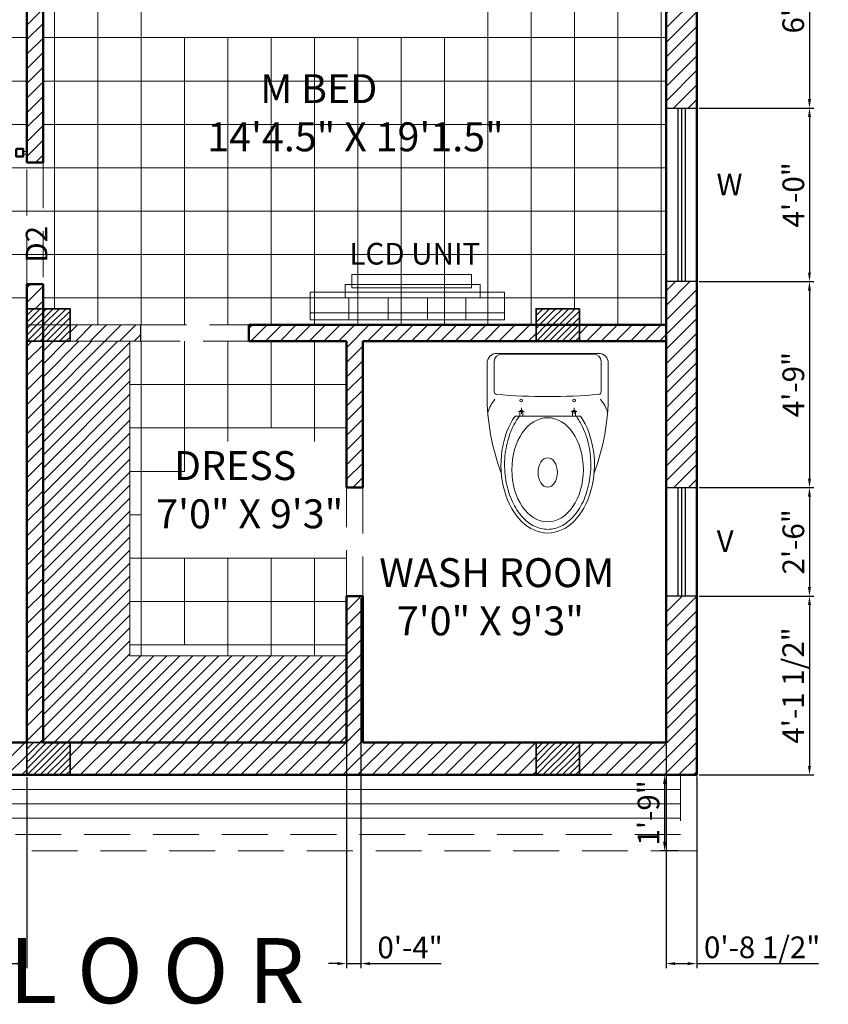
# Model space of a CAD drawing. Units: millimetres. Extents: x 225995 to 227247, y 225507 to 226008.
# Tile 4 of 23: x 226378 to 226602, y 225507 to 225780. Entities that reach past the tile are written whole.
import ezdxf

# ---------------------------------------------------------------- set-up
doc = ezdxf.new("R2010")
doc.units = ezdxf.units.MM
doc.linetypes.add('DASHED', pattern=[19.05, 12.7, -6.35])
for name, color, linetype, lineweight in [('A-ANNO-DIMS', 2, 'Continuous', 18), ('A-ANNO-TEXT', 3, 'Continuous', 18), ('A-AREA-IDEN', 30, 'Continuous', 18), ('A-COLS', 40, 'Continuous', 35), ('A-FLOR-FIXT', 8, 'Continuous', 18), ('A-FLOR-PATT', 8, 'Continuous', 13), ('A-FURN', 9, 'Continuous', 18), ('A-GLAZ', 4, 'Continuous', 25), ('A-WALL', 7, 'Continuous', 50), ('A-WALL-OVHD', 1, 'DASHED', 18), ('A-WALL-PATT', 8, 'Continuous', 13)]:
    doc.layers.add(name, color=color, linetype=linetype, lineweight=lineweight)
doc.styles.get("Standard").update_dxf_attribs({"font": 'arial.ttf'})
doc.dimstyles.new('ISO-25', dxfattribs={"dimtxt": 6, "dimasz": 2.5, "dimexe": 1.25, "dimexo": 0.625, "dimtad": 1, "dimdec": 0, "dimlunit": 3, "dimtxsty": 'Standard', "dimcen": 2.5, "dimadec": 0, "dimazin": 0, "dimtfac": 1, "dimtdec": 0, "dimtmove": 0, "dimatfit": 3, "dimfxl": 1, "dimarcsym": 0})
pattern_1 = [(45, (141, 0), (-0.898025612, 0.898025612), [])]
pattern_2 = [(45, (0, -120), (-0.898025612, 0.898025612), [])]
pattern_3 = [(45, (141, -120), (-0.898025612, 0.898025612), [])]

# ---------------------------------------------------------------- blocks, each defined once
blk = doc.blocks.new('A$C005B7AE8')
for p, q in [((0.46, 0.74), (0.04, 0.74)), ((0.44, 0.7369), (0.06, 0.7369)), ((0, 0.7), (0, 0.569)), ((0.03, 0.7069), (0.03, 0.5811)), ((0.47, 0.7069), (0.47, 0.5811)), ((0.5, 0.7), (0.5, 0.569)), ((0.1298, 0.5004), (0.1534, 0.5004)), ((0.1356, 0.482), (0.1356, 0.5012)), ((0.1415, 0.4917), (0.1415, 0.5154)), ((0.1478, 0.5012), (0.1478, 0.482)), ((0.3702, 0.5004), (0.3466, 0.5004)), ((0.3522, 0.5012), (0.3522, 0.482)), ((0.3585, 0.4917), (0.3585, 0.5154)), ((0.3644, 0.482), (0.3644, 0.5012)), ((0.3847, 0.482), (0.1153, 0.482))]:
    blk.add_line(p, q)
for centre in [(0.1408, 0.546), (0.3592, 0.546)]:
    blk.add_circle(centre, 0.00582)
for centre, radius, start, end in [((0.04, 0.7), 0.04, 90, 180), ((0.06, 0.7069), 0.03, 90, 180), ((0.44, 0.7069), 0.03, 0, 90), ((0.46, 0.7), 0.04, 0, 90), ((0.9162, 0.5698), 0.9162, 179.9528, 200.6123), ((0.04, 0.5811), 0.01, 180, 265.0115), ((0.25, 2.987), 2.425, 265.0115, 274.9885), ((-0.4162, 0.5698), 0.9162, 339.3877, 0.0472), ((0.46, 0.5811), 0.01, 274.9885, 0), ((0.1538, 0.4498), 0.1579, 140.1815, 162.8478), ((0.3462, 0.4498), 0.1579, 17.1522, 39.8185), ((0.1417, 0.5006), 0.00615, 5.1568, 174.8432), ((0.3583, 0.5006), 0.00615, 5.1568, 174.8432)]:
    blk.add_arc(centre, radius, start, end)
blk.add_ellipse((0.25, 0.281), major_axis=(0, -0.281), ratio=0.685919, start_param=3.915332, end_param=8.651039)
for centre, major_axis, ratio in [((0.2497, 0.2607), (0, -0.2144), 0.687861), ((0.25, 0.2496), (0, -0.0607), 0.657164)]:
    blk.add_ellipse(centre, major_axis=major_axis, ratio=ratio)
blk.add_open_spline([(0.133, 0.4806), (0.1233, 0.4673), (0.1192, 0.4608), (0.109, 0.4431), (0.1032, 0.4313), (0.0931, 0.4064), (0.0887, 0.3933), (0.0814, 0.3662), (0.0785, 0.3521), (0.0743, 0.3236), (0.073, 0.3091), (0.072, 0.2798), (0.0723, 0.2652), (0.0746, 0.2361), (0.0765, 0.2217), (0.0819, 0.1936), (0.0854, 0.1799), (0.0938, 0.1536), (0.0988, 0.141), (0.1099, 0.1171), (0.1162, 0.1059), (0.1297, 0.0851), (0.137, 0.0756), (0.1525, 0.0585), (0.1607, 0.0509), (0.1776, 0.0379), (0.1863, 0.0325), (0.2042, 0.0237), (0.2132, 0.0204), (0.2316, 0.0161), (0.2408, 0.015), (0.2593, 0.015), (0.2685, 0.0161), (0.2868, 0.0205), (0.2959, 0.0237), (0.3137, 0.0325), (0.3225, 0.0379), (0.3394, 0.051), (0.3475, 0.0586), (0.363, 0.0756), (0.3703, 0.0852), (0.3839, 0.1059), (0.3901, 0.1172), (0.4013, 0.141), (0.4062, 0.1537), (0.4146, 0.18), (0.4181, 0.1937), (0.4235, 0.2218), (0.4255, 0.2362), (0.4277, 0.2653), (0.428, 0.2799), (0.427, 0.3091), (0.4257, 0.3237), (0.4215, 0.3522), (0.4186, 0.3662), (0.4113, 0.3933), (0.4069, 0.4064), (0.3967, 0.4313), (0.391, 0.4432), (0.3808, 0.4609), (0.3767, 0.4673), (0.3673, 0.4823)], degree=3, knots=[3.915332, 3.915332, 3.915332, 3.915332, 4.014441, 4.014441, 4.176505, 4.176505, 4.338569, 4.338569, 4.500633, 4.500633, 4.662697, 4.662697, 4.824761, 4.824761, 4.986825, 4.986825, 5.148889, 5.148889, 5.310953, 5.310953, 5.473017, 5.473017, 5.635081, 5.635081, 5.797146, 5.797146, 5.95921, 5.95921, 6.121274, 6.121274, 6.283338, 6.283338, 6.445402, 6.445402, 6.607466, 6.607466, 6.76953, 6.76953, 6.931594, 6.931594, 7.093658, 7.093658, 7.255722, 7.255722, 7.417786, 7.417786, 7.57985, 7.57985, 7.741915, 7.741915, 7.903979, 7.903979, 8.066043, 8.066043, 8.228107, 8.228107, 8.390171, 8.390171, 8.552235, 8.552235, 8.651039, 8.651039, 8.651039, 8.651039])
blk = doc.blocks.new('*D67')
at = {"layer": 'A-ANNO-DIMS', "color": 0, "lineweight": -2, "transparency": 16777216}
for p, q in [((226560.75, 225570.77), (226555.72, 225570.77)), ((226556.97, 225568.27), (226556.97, 225552.27)), ((226560.75, 225549.77), (226555.72, 225549.77))]:
    blk.add_line(p, q, dxfattribs=at)
at = {"layer": 'A-ANNO-DIMS', "color": 0, "transparency": 16777216}
for points in [[(226556.55, 225568.27), (226557.38, 225568.27), (226556.97, 225570.77)], [(226556.55, 225552.27), (226557.38, 225552.27), (226556.97, 225549.77)]]:
    blk.add_solid(points, dxfattribs=at)
at = {"layer": 'Defpoints', "color": 0, "transparency": 16777216}
for p in [(226561.38, 225570.77), (226556.97, 225549.77), (226561.38, 225549.77)]:
    blk.add_point(p, dxfattribs=at)
at = {"layer": 'A-ANNO-DIMS', "color": 0, "transparency": 16777216, "insert": (226553.28, 225560.27), "char_height": 6, "attachment_point": 5, "rotation": 90}
blk.add_mtext('1\'-9"', dxfattribs=at)
blk = doc.blocks.new('*D91')
at = {"layer": 'A-ANNO-DIMS', "color": 0, "lineweight": -2, "transparency": 16777216}
for p, q in [((226557.38, 225579.15), (226557.38, 225517.32)), ((226565.88, 225570.15), (226565.88, 225517.32)), ((226559.88, 225518.57), (226563.38, 225518.57)), ((226565.88, 225518.57), (226599.56, 225518.57))]:
    blk.add_line(p, q, dxfattribs=at)
at = {"layer": 'A-ANNO-DIMS', "color": 0, "transparency": 16777216}
for points in [[(226559.88, 225518.99), (226559.88, 225518.16), (226557.38, 225518.57)], [(226563.38, 225518.99), (226563.38, 225518.16), (226565.88, 225518.57)]]:
    blk.add_solid(points, dxfattribs=at)
at = {"layer": 'Defpoints', "color": 0, "transparency": 16777216}
for p in [(226557.38, 225579.77), (226565.88, 225570.77), (226565.88, 225518.57)]:
    blk.add_point(p, dxfattribs=at)
at = {"layer": 'A-ANNO-DIMS', "color": 0, "transparency": 16777216, "insert": (226583.97, 225522.3), "char_height": 6, "attachment_point": 5}
blk.add_mtext('0\'-8 1/2"', dxfattribs=at)
blk = doc.blocks.new('*D92')
at = {"layer": 'A-ANNO-DIMS', "color": 0, "lineweight": -2, "transparency": 16777216}
for p, q in [((226468.88, 225619.65), (226468.88, 225517.32)), ((226472.89, 225619.65), (226472.89, 225517.32)), ((226466.38, 225518.57), (226463.88, 225518.57)), ((226468.88, 225518.57), (226472.89, 225518.57)), ((226475.39, 225518.57), (226495.09, 225518.57))]:
    blk.add_line(p, q, dxfattribs=at)
at = {"layer": 'A-ANNO-DIMS', "color": 0, "transparency": 16777216}
for points in [[(226466.38, 225518.99), (226466.38, 225518.16), (226468.88, 225518.57)], [(226475.39, 225518.99), (226475.39, 225518.16), (226472.89, 225518.57)]]:
    blk.add_solid(points, dxfattribs=at)
at = {"layer": 'Defpoints', "color": 0, "transparency": 16777216}
for p in [(226468.88, 225620.27), (226472.89, 225620.27), (226472.89, 225518.57)]:
    blk.add_point(p, dxfattribs=at)
at = {"layer": 'A-ANNO-DIMS', "color": 0, "transparency": 16777216, "insert": (226486.49, 225522.26), "char_height": 6, "attachment_point": 5}
blk.add_mtext('0\'-4"', dxfattribs=at)
blk = doc.blocks.new('*D101')
at = {"layer": 'A-ANNO-DIMS', "color": 0, "lineweight": -2, "transparency": 16777216}
for p, q in [((226566.5, 225828.77), (226598.33, 225828.77)), ((226597.08, 225826.27), (226597.08, 225757.77)), ((226566.5, 225755.27), (226598.33, 225755.27))]:
    blk.add_line(p, q, dxfattribs=at)
at = {"layer": 'A-ANNO-DIMS', "color": 0, "transparency": 16777216}
for points in [[(226596.66, 225826.27), (226597.49, 225826.27), (226597.08, 225828.77)], [(226596.66, 225757.77), (226597.49, 225757.77), (226597.08, 225755.27)]]:
    blk.add_solid(points, dxfattribs=at)
at = {"layer": 'Defpoints', "color": 0, "transparency": 16777216}
for p in [(226565.88, 225828.77), (226565.88, 225755.27), (226597.08, 225755.27)]:
    blk.add_point(p, dxfattribs=at)
at = {"layer": 'A-ANNO-DIMS', "color": 0, "transparency": 16777216, "insert": (226593.35, 225792.02), "char_height": 6, "attachment_point": 5, "rotation": 90}
blk.add_mtext('6\'-1 1/2"', dxfattribs=at)
blk = doc.blocks.new('*D102')
at = {"layer": 'A-ANNO-DIMS', "color": 0, "lineweight": -2, "transparency": 16777216}
for p, q in [((226566.5, 225755.27), (226598.33, 225755.27)), ((226597.08, 225752.77), (226597.08, 225709.77)), ((226566.5, 225707.27), (226598.33, 225707.27))]:
    blk.add_line(p, q, dxfattribs=at)
at = {"layer": 'A-ANNO-DIMS', "color": 0, "transparency": 16777216}
for points in [[(226596.66, 225752.77), (226597.49, 225752.77), (226597.08, 225755.27)], [(226596.66, 225709.77), (226597.49, 225709.77), (226597.08, 225707.27)]]:
    blk.add_solid(points, dxfattribs=at)
at = {"layer": 'Defpoints', "color": 0, "transparency": 16777216}
for p in [(226565.88, 225755.27), (226565.88, 225707.27), (226597.08, 225707.27)]:
    blk.add_point(p, dxfattribs=at)
at = {"layer": 'A-ANNO-DIMS', "color": 0, "transparency": 16777216, "insert": (226593.39, 225731.27), "char_height": 6, "attachment_point": 5, "rotation": 90}
blk.add_mtext('4\'-0"', dxfattribs=at)
blk = doc.blocks.new('*D103')
at = {"layer": 'A-ANNO-DIMS', "color": 0, "lineweight": -2, "transparency": 16777216}
for p, q in [((226566.5, 225707.27), (226598.33, 225707.27)), ((226597.08, 225704.77), (226597.08, 225652.77)), ((226566.5, 225650.27), (226598.33, 225650.27))]:
    blk.add_line(p, q, dxfattribs=at)
at = {"layer": 'A-ANNO-DIMS', "color": 0, "transparency": 16777216}
for points in [[(226596.66, 225704.77), (226597.49, 225704.77), (226597.08, 225707.27)], [(226596.66, 225652.77), (226597.49, 225652.77), (226597.08, 225650.27)]]:
    blk.add_solid(points, dxfattribs=at)
at = {"layer": 'Defpoints', "color": 0, "transparency": 16777216}
for p in [(226565.88, 225707.27), (226565.88, 225650.27), (226597.08, 225650.27)]:
    blk.add_point(p, dxfattribs=at)
at = {"layer": 'A-ANNO-DIMS', "color": 0, "transparency": 16777216, "insert": (226593.39, 225678.77), "char_height": 6, "attachment_point": 5, "rotation": 90}
blk.add_mtext('4\'-9"', dxfattribs=at)
blk = doc.blocks.new('*D104')
at = {"layer": 'A-ANNO-DIMS', "color": 0, "lineweight": -2, "transparency": 16777216}
for p, q in [((226566.5, 225650.27), (226598.33, 225650.27)), ((226597.08, 225647.77), (226597.08, 225622.77)), ((226566.5, 225620.27), (226598.33, 225620.27))]:
    blk.add_line(p, q, dxfattribs=at)
at = {"layer": 'A-ANNO-DIMS', "color": 0, "transparency": 16777216}
for points in [[(226596.66, 225647.77), (226597.49, 225647.77), (226597.08, 225650.27)], [(226596.66, 225622.77), (226597.49, 225622.77), (226597.08, 225620.27)]]:
    blk.add_solid(points, dxfattribs=at)
at = {"layer": 'Defpoints', "color": 0, "transparency": 16777216}
for p in [(226565.88, 225650.27), (226565.88, 225620.27), (226597.08, 225620.27)]:
    blk.add_point(p, dxfattribs=at)
at = {"layer": 'A-ANNO-DIMS', "color": 0, "transparency": 16777216, "insert": (226593.39, 225635.27), "char_height": 6, "attachment_point": 5, "rotation": 90}
blk.add_mtext('2\'-6"', dxfattribs=at)
blk = doc.blocks.new('*D105')
at = {"layer": 'A-ANNO-DIMS', "color": 0, "lineweight": -2, "transparency": 16777216}
for p, q in [((226566.5, 225620.27), (226598.33, 225620.27)), ((226597.08, 225617.77), (226597.08, 225573.27)), ((226566.5, 225570.77), (226598.33, 225570.77))]:
    blk.add_line(p, q, dxfattribs=at)
at = {"layer": 'A-ANNO-DIMS', "color": 0, "transparency": 16777216}
for points in [[(226596.66, 225617.77), (226597.49, 225617.77), (226597.08, 225620.27)], [(226596.66, 225573.27), (226597.49, 225573.27), (226597.08, 225570.77)]]:
    blk.add_solid(points, dxfattribs=at)
at = {"layer": 'Defpoints', "color": 0, "transparency": 16777216}
for p in [(226565.88, 225620.27), (226565.88, 225570.77), (226597.08, 225570.77)]:
    blk.add_point(p, dxfattribs=at)
at = {"layer": 'A-ANNO-DIMS', "color": 0, "transparency": 16777216, "insert": (226593.35, 225595.52), "char_height": 6, "attachment_point": 5, "rotation": 90}
blk.add_mtext('4\'-1 1/2"', dxfattribs=at)
blk = doc.blocks.new('*D107')
at = {"layer": 'A-ANNO-DIMS', "color": 0, "lineweight": -2, "transparency": 16777216}
for p, q in [((226344.38, 225570.15), (226344.38, 225517.32)), ((226380.38, 225570.15), (226380.38, 225517.32)), ((226346.88, 225518.57), (226377.88, 225518.57))]:
    blk.add_line(p, q, dxfattribs=at)
at = {"layer": 'A-ANNO-DIMS', "color": 0, "transparency": 16777216}
for points in [[(226346.88, 225518.99), (226346.88, 225518.16), (226344.38, 225518.57)], [(226377.88, 225518.99), (226377.88, 225518.16), (226380.38, 225518.57)]]:
    blk.add_solid(points, dxfattribs=at)
at = {"layer": 'Defpoints', "color": 0, "transparency": 16777216}
for p in [(226344.38, 225570.77), (226380.38, 225570.77), (226380.38, 225518.57)]:
    blk.add_point(p, dxfattribs=at)
at = {"layer": 'A-ANNO-DIMS', "color": 0, "transparency": 16777216, "insert": (226362.38, 225522.26), "char_height": 6, "attachment_point": 5}
blk.add_mtext('3\'-0"', dxfattribs=at)

msp = doc.modelspace()

# ---------------------------------------------------------------- hatches: boundary and pattern name
at = {"layer": 'A-WALL-PATT'}
h = msp.add_hatch(dxfattribs=at)
h.set_pattern_fill('ANSI31', color=256, scale=0.9)
h.paths.add_polyline_path([(226565.88, 225828.77), (226557.38, 225828.77), (226557.38, 225755.27), (226565.88, 225755.27)])
h = msp.add_hatch(dxfattribs=at)
h.set_pattern_fill('ANSI31', color=256, scale=0.9)
h.paths.add_polyline_path([(226384.88, 225808.91), (226380.38, 225808.91), (226380.38, 225740.27), (226384.88, 225740.27)])
h = msp.add_hatch(dxfattribs=at)
h.set_pattern_fill('ANSI31', color=256, scale=0.9)
h.paths.add_polyline_path([(226565.88, 225707.27), (226557.38, 225707.27), (226557.38, 225695.27), (226533.38, 225695.27), (226533.38, 225690.77), (226557.38, 225690.77), (226557.38, 225650.27), (226565.88, 225650.27)])
h = msp.add_hatch(dxfattribs=at)
h.set_pattern_fill('ANSI31', color=256, scale=0.9)
h.paths.add_polyline_path([(226384.88, 225706.52), (226380.38, 225706.52), (226380.38, 225699.77), (226384.88, 225699.77)])
h = msp.add_hatch(dxfattribs=at)
h.set_pattern_fill('ANSI31', color=256, scale=0.4)
h.paths.add_polyline_path([(226384.88, 225699.77), (226380.38, 225699.77), (226380.38, 225695.27), (226384.88, 225695.27)])
h = msp.add_hatch(dxfattribs=at)
h.set_pattern_fill('ANSI31', color=256, scale=0.4)
h.paths.add_polyline_path([(226392.38, 225699.77), (226384.88, 225699.77), (226384.88, 225695.27), (226392.38, 225695.27)])
h = msp.add_hatch(dxfattribs=at)
h.set_pattern_fill('ANSI31', color=256, scale=0.4)
h.set_pattern_definition(pattern_1)
h.paths.add_polyline_path([(226525.88, 225699.77), (226521.38, 225699.77), (226521.38, 225695.27), (226525.88, 225695.27)])
h = msp.add_hatch(dxfattribs=at)
h.set_pattern_fill('ANSI31', color=256, scale=0.4)
h.set_pattern_definition(pattern_1)
h.paths.add_polyline_path([(226533.38, 225699.77), (226525.88, 225699.77), (226525.88, 225695.27), (226533.38, 225695.27)])
h = msp.add_hatch(dxfattribs=at)
h.set_pattern_fill('ANSI31', color=256, scale=0.4)
h.paths.add_polyline_path([(226384.88, 225695.27), (226380.38, 225695.27), (226380.38, 225690.77), (226384.88, 225690.77)])
h = msp.add_hatch(dxfattribs=at)
h.set_pattern_fill('ANSI31', color=256, scale=0.4)
h.paths.add_polyline_path([(226392.38, 225695.27), (226384.88, 225695.27), (226384.88, 225690.77), (226392.38, 225690.77)])
h = msp.add_hatch(dxfattribs=at)
h.set_pattern_fill('ANSI31', color=256, scale=0.9)
h.paths.add_polyline_path([(226411.88, 225695.27), (226392.38, 225695.27), (226392.38, 225690.77), (226411.88, 225690.77)])
h = msp.add_hatch(dxfattribs=at)
h.set_pattern_fill('ANSI31', color=256, scale=0.9)
h.paths.add_polyline_path([(226521.38, 225695.27), (226441.88, 225695.27), (226441.88, 225690.77), (226468.88, 225690.77), (226468.88, 225650.27), (226473.38, 225650.27), (226473.38, 225690.77), (226521.38, 225690.77)])
h = msp.add_hatch(dxfattribs=at)
h.set_pattern_fill('ANSI31', color=256, scale=0.4)
h.set_pattern_definition(pattern_1)
h.paths.add_polyline_path([(226525.88, 225695.27), (226521.38, 225695.27), (226521.38, 225690.77), (226525.88, 225690.77)])
h = msp.add_hatch(dxfattribs=at)
h.set_pattern_fill('ANSI31', color=256, scale=0.4)
h.set_pattern_definition(pattern_1)
h.paths.add_polyline_path([(226533.38, 225695.27), (226525.88, 225695.27), (226525.88, 225690.77), (226533.38, 225690.77)])
h = msp.add_hatch(dxfattribs=at)
h.set_pattern_fill('ANSI31', color=256, scale=0.9)
h.paths.add_polyline_path([(226384.88, 225690.77), (226380.38, 225690.77), (226380.38, 225579.77), (226384.88, 225579.77)])
h = msp.add_hatch(dxfattribs=at)
h.set_pattern_fill('ANSI31', color=256, scale=0.8)
h.paths.add_polyline_path([(226468.88, 225603.77), (226408.88, 225603.77), (226408.88, 225690.77), (226384.88, 225690.77), (226384.88, 225579.77), (226392.38, 225579.77), (226468.88, 225579.77)])
h = msp.add_hatch(dxfattribs=at)
h.set_pattern_fill('ANSI31', color=256, scale=0.9)
h.paths.add_polyline_path([(226521.38, 225579.77), (226473.38, 225579.77), (226473.38, 225620.27), (226468.88, 225620.27), (226468.88, 225579.77), (226392.38, 225579.77), (226392.38, 225570.77), (226521.38, 225570.77)])
h = msp.add_hatch(dxfattribs=at)
h.set_pattern_fill('ANSI31', color=256, scale=0.9)
h.paths.add_polyline_path([(226565.88, 225620.27), (226557.38, 225620.27), (226557.38, 225579.77), (226533.38, 225579.77), (226533.38, 225570.77), (226565.88, 225570.77)])
h = msp.add_hatch(dxfattribs=at)
h.set_pattern_fill('ANSI31', color=256, scale=0.9)
h.paths.add_polyline_path([(226380.38, 225579.77), (226344.38, 225579.77), (226344.38, 225570.77), (226380.38, 225570.77)])
h = msp.add_hatch(dxfattribs=at)
h.set_pattern_fill('ANSI31', color=256, scale=0.4)
h.set_pattern_definition(pattern_2)
h.paths.add_polyline_path([(226384.88, 225579.77), (226380.38, 225579.77), (226380.38, 225575.27), (226384.88, 225575.27)])
h = msp.add_hatch(dxfattribs=at)
h.set_pattern_fill('ANSI31', color=256, scale=0.4)
h.set_pattern_definition(pattern_2)
h.paths.add_polyline_path([(226392.38, 225579.77), (226384.88, 225579.77), (226384.88, 225575.27), (226392.38, 225575.27)])
h = msp.add_hatch(dxfattribs=at)
h.set_pattern_fill('ANSI31', color=256, scale=0.4)
h.set_pattern_definition(pattern_3)
h.paths.add_polyline_path([(226525.88, 225579.77), (226521.38, 225579.77), (226521.38, 225575.27), (226525.88, 225575.27)])
h = msp.add_hatch(dxfattribs=at)
h.set_pattern_fill('ANSI31', color=256, scale=0.4)
h.set_pattern_definition(pattern_3)
h.paths.add_polyline_path([(226533.38, 225579.77), (226525.88, 225579.77), (226525.88, 225575.27), (226533.38, 225575.27)])
h = msp.add_hatch(dxfattribs=at)
h.set_pattern_fill('ANSI31', color=256, scale=0.4)
h.set_pattern_definition(pattern_2)
h.paths.add_polyline_path([(226384.88, 225575.27), (226380.38, 225575.27), (226380.38, 225570.77), (226384.88, 225570.77)])
h = msp.add_hatch(dxfattribs=at)
h.set_pattern_fill('ANSI31', color=256, scale=0.4)
h.set_pattern_definition(pattern_2)
h.paths.add_polyline_path([(226392.38, 225575.27), (226384.88, 225575.27), (226384.88, 225570.77), (226392.38, 225570.77)])
h = msp.add_hatch(dxfattribs=at)
h.set_pattern_fill('ANSI31', color=256, scale=0.4)
h.set_pattern_definition(pattern_3)
h.paths.add_polyline_path([(226525.88, 225575.27), (226521.38, 225575.27), (226521.38, 225570.77), (226525.88, 225570.77)])
h = msp.add_hatch(dxfattribs=at)
h.set_pattern_fill('ANSI31', color=256, scale=0.4)
h.set_pattern_definition(pattern_3)
h.paths.add_polyline_path([(226533.38, 225575.27), (226525.88, 225575.27), (226525.88, 225570.77), (226533.38, 225570.77)])

# ---------------------------------------------------------------- linework, layer by layer
at = {"layer": 'A-ANNO-TEXT'}
msp.add_line((226424.05, 225630.77), (226424.05, 225606.77), dxfattribs=at)
at = {"layer": 'A-COLS'}
for points in [[(226380.38, 225690.77), (226380.38, 225699.77), (226392.38, 225699.77), (226392.38, 225690.77)], [(226521.38, 225690.77), (226521.38, 225699.77), (226533.38, 225699.77), (226533.38, 225690.77)], [(226380.38, 225570.77), (226380.38, 225579.77), (226392.38, 225579.77), (226392.38, 225570.77)], [(226521.38, 225570.77), (226521.38, 225579.77), (226533.38, 225579.77), (226533.38, 225570.77)]]:
    msp.add_lwpolyline(points, close=True, dxfattribs=at)
at = {"layer": 'A-FLOR-PATT'}
for p, q in [((226400.05, 225900.77), (226400.05, 225695.27)), ((226412.05, 225900.77), (226412.05, 225695.27)), ((226508.05, 225900.77), (226508.05, 225695.27)), ((226520.05, 225900.77), (226520.05, 225695.27)), ((226532.05, 225900.77), (226532.05, 225699.77)), ((226544.05, 225900.77), (226544.05, 225695.27)), ((226388.05, 225808.91), (226388.05, 225699.77)), ((226219.88, 225774.77), (226380.38, 225774.77)), ((226384.88, 225774.77), (226557.38, 225774.77)), ((226424.05, 225774.77), (226424.05, 225695.27)), ((226436.05, 225774.77), (226436.05, 225695.27)), ((226448.05, 225774.77), (226448.05, 225695.27)), ((226460.05, 225774.77), (226460.05, 225695.27)), ((226472.05, 225774.77), (226472.05, 225695.27)), ((226484.05, 225774.77), (226484.05, 225695.27)), ((226496.05, 225774.77), (226496.05, 225695.27)), ((226219.88, 225762.77), (226380.38, 225762.77)), ((226384.88, 225762.77), (226557.38, 225762.77)), ((226219.88, 225750.77), (226380.38, 225750.77)), ((226384.88, 225750.77), (226557.38, 225750.77)), ((226111.88, 225738.77), (226557.38, 225738.77)), ((226111.88, 225726.77), (226557.38, 225726.77)), ((226111.88, 225714.77), (226557.38, 225714.77)), ((226111.88, 225702.77), (226380.38, 225702.77)), ((226384.88, 225702.77), (226557.38, 225702.77)), ((226038.38, 225566.77), (226561.38, 225566.77)), ((226038.38, 225562.77), (226561.38, 225562.77)), ((226038.38, 225558.77), (226561.38, 225558.77))]:
    msp.add_line(p, q, dxfattribs=at)
at = {"layer": 'A-FURN'}
for p, q in [((226556.05, 225900.77), (226556.05, 225695.27)), ((226557.38, 225755.27), (226565.88, 225755.27)), ((226379.39, 225743.31), (226380.38, 225743.31)), ((226379.39, 225742.52), (226380.38, 225742.52)), ((226557.38, 225707.27), (226565.88, 225707.27)), ((226469.56, 225702.77), (226469.56, 225696.67)), ((226480.47, 225702.77), (226480.47, 225699.61)), ((226491.33, 225702.77), (226491.33, 225696.67)), ((226501.9, 225702.77), (226501.9, 225696.67)), ((226458.85, 225698.62), (226512.66, 225698.62)), ((226480.47, 225699.61), (226480.47, 225696.67)), ((226380.38, 225695.27), (226411.88, 225695.27)), ((226392.38, 225695.27), (226411.92, 225695.27)), ((226411.88, 225690.77), (226411.88, 225695.27)), ((226411.92, 225695.27), (226411.88, 225690.77)), ((226384.88, 225690.77), (226411.88, 225690.77)), ((226411.88, 225690.77), (226384.88, 225690.77)), ((226408.88, 225603.77), (226408.88, 225690.77)), ((226412.05, 225690.77), (226412.05, 225603.77)), ((226424.05, 225690.77), (226424.05, 225654.77)), ((226436.05, 225690.77), (226436.05, 225663.02)), ((226448.05, 225690.77), (226448.05, 225666.77)), ((226460.05, 225690.77), (226460.05, 225663.02)), ((226408.88, 225678.77), (226468.88, 225678.77)), ((226408.88, 225666.77), (226468.88, 225666.77)), ((226408.88, 225654.77), (226424.05, 225654.77)), ((226557.38, 225650.27), (226565.88, 225650.27)), ((226408.88, 225642.77), (226412.05, 225642.77)), ((226408.88, 225630.77), (226468.88, 225630.77)), ((226436.05, 225630.77), (226436.05, 225603.77)), ((226448.05, 225630.77), (226448.05, 225603.77)), ((226460.05, 225630.77), (226460.05, 225603.77)), ((226557.38, 225620.27), (226565.88, 225620.27)), ((226408.88, 225618.77), (226468.88, 225618.77)), ((226408.88, 225606.77), (226468.88, 225606.77)), ((226408.88, 225603.77), (226468.88, 225603.77))]:
    msp.add_line(p, q, dxfattribs=at)
for points in [[(226470.39, 225709.24), (226503.47, 225709.24), (226503.47, 225705.58), (226470.39, 225705.58)], [(226458.85, 225704.36), (226512.66, 225704.36), (226512.66, 225696.67), (226458.85, 225696.67)], [(226468.51, 225706.47), (226505.92, 225706.47), (226505.92, 225702.77), (226468.51, 225702.77)]]:
    msp.add_lwpolyline(points, close=True, dxfattribs=at)
at = {"layer": 'A-GLAZ'}
for p, q in [((226560.63, 225755.27), (226560.63, 225707.27)), ((226561.63, 225755.27), (226561.63, 225707.27)), ((226562.63, 225755.27), (226562.63, 225707.27)), ((226560.63, 225650.27), (226560.63, 225620.27)), ((226561.63, 225650.27), (226561.63, 225620.27)), ((226562.63, 225650.27), (226562.63, 225620.27))]:
    msp.add_line(p, q, dxfattribs=at)
for points in [[(226557.38, 225755.27), (226565.88, 225755.27), (226565.88, 225707.27), (226557.38, 225707.27)], [(226557.38, 225650.27), (226565.88, 225650.27), (226565.88, 225620.27), (226557.38, 225620.27)]]:
    msp.add_lwpolyline(points, close=True, dxfattribs=at)
at = {"layer": 'A-WALL'}
for p, q in [((226565.88, 225933.77), (226565.88, 225570.77)), ((226565.88, 225570.77), (226565.88, 225933.77)), ((226380.38, 225740.27), (226380.38, 225924.77)), ((226380.38, 225924.77), (226380.38, 225740.27)), ((226384.88, 225740.27), (226384.88, 225924.77)), ((226384.88, 225740.27), (226384.88, 225924.77)), ((226557.38, 225695.27), (226557.38, 225924.77)), ((226557.38, 225924.77), (226557.38, 225579.77)), ((226380.38, 225740.27), (226384.88, 225740.27)), ((226380.38, 225740.27), (226384.88, 225740.27)), ((226380.38, 225579.77), (226380.38, 225706.52)), ((226380.38, 225706.52), (226384.88, 225706.52)), ((226384.88, 225706.52), (226380.38, 225706.52)), ((226380.38, 225706.52), (226380.38, 225579.77)), ((226384.88, 225695.27), (226384.88, 225706.52)), ((226384.88, 225579.77), (226384.88, 225706.52)), ((226384.88, 225579.77), (226384.88, 225695.27)), ((226441.88, 225690.77), (226441.88, 225695.27)), ((226441.88, 225695.27), (226557.38, 225695.27)), ((226441.88, 225695.27), (226557.38, 225695.27)), ((226441.88, 225690.77), (226441.88, 225695.27)), ((226557.38, 225695.27), (226557.38, 225690.77)), ((226441.88, 225690.77), (226468.88, 225690.77)), ((226468.88, 225690.77), (226441.88, 225690.77)), ((226468.88, 225650.27), (226468.88, 225690.77)), ((226468.88, 225650.27), (226468.88, 225690.77)), ((226473.38, 225690.77), (226557.38, 225690.77)), ((226473.38, 225650.27), (226473.38, 225690.77)), ((226557.38, 225690.77), (226473.38, 225690.77)), ((226473.38, 225690.77), (226473.38, 225650.27)), ((226557.38, 225579.77), (226557.38, 225690.77)), ((226468.88, 225650.27), (226473.38, 225650.27)), ((226473.38, 225650.27), (226468.88, 225650.27)), ((226468.88, 225579.77), (226468.88, 225620.27)), ((226468.88, 225620.27), (226473.38, 225620.27)), ((226472.89, 225620.27), (226468.88, 225620.27)), ((226473.38, 225620.27), (226468.88, 225620.27)), ((226468.88, 225620.27), (226468.88, 225579.77)), ((226473.38, 225579.77), (226473.38, 225620.27)), ((226473.38, 225579.77), (226473.38, 225620.27)), ((226380.38, 225579.77), (226111.88, 225579.77)), ((226344.38, 225579.77), (226380.38, 225579.77)), ((226384.88, 225579.77), (226468.88, 225579.77)), ((226468.88, 225579.77), (226384.88, 225579.77)), ((226473.38, 225579.77), (226557.38, 225579.77)), ((226557.38, 225579.77), (226473.38, 225579.77)), ((226102.88, 225570.77), (226565.88, 225570.77)), ((226344.38, 225570.77), (226565.88, 225570.77))]:
    msp.add_line(p, q, dxfattribs=at)
msp.add_lwpolyline([(226377.42, 225743.99), (226379.39, 225743.99), (226379.39, 225741.91), (226377.42, 225741.91)], close=True, dxfattribs=at)
at = {"layer": 'A-WALL-OVHD'}
for p, q in [((226561.38, 225570.77), (226561.38, 225554.27)), ((226565.88, 225570.77), (226565.88, 225549.77)), ((226561.38, 225554.27), (226038.38, 225554.27)), ((226565.88, 225549.77), (226033.88, 225549.77))]:
    msp.add_line(p, q, dxfattribs=at)
for points in [[(226380.38, 225740.27), (226384.88, 225740.27), (226384.88, 225706.52), (226380.38, 225706.52)], [(226411.92, 225695.27), (226441.88, 225695.27), (226441.88, 225690.77), (226411.92, 225690.77)], [(226468.88, 225650.27), (226473.38, 225650.27), (226473.38, 225620.27), (226468.88, 225620.27)]]:
    msp.add_lwpolyline(points, close=True, dxfattribs=at)

# ---------------------------------------------------------------- block references
at = {"layer": 'A-FLOR-FIXT', "xscale": 67.15513792430541, "yscale": 67.15513792430541, "zscale": 67.15513792430541}
msp.add_blockref('A$C005B7AE8', (226507.81, 225637.71), dxfattribs=at)

# ---------------------------------------------------------------- texts
at = {"layer": 'A-ANNO-TEXT', "attachment_point": 1}
for s, width, insert, char_height in [('   W', 24.8115, (226565.85, 225737.13), 6), ('   LCD UNIT', 85.4795, (226464.18, 225717.99), 6), ('   V', 24.8115, (226565.88, 225638.49), 6), ('D U P L E X  SECOND F L O O R', 408.2479, (226122.73, 225525.63), 18)]:
    msp.add_mtext_dynamic_manual_height_columns(s, width=width, gutter_width=12.5, heights=[0], dxfattribs=dict(at, insert=insert, char_height=char_height))
at = {"layer": 'A-ANNO-TEXT', "insert": (226380.09, 225712.51), "char_height": 6, "attachment_point": 1, "rotation": 90}
msp.add_mtext_dynamic_manual_height_columns('D2', width=8.157, gutter_width=12.5, heights=[0], dxfattribs=at)
at = {"layer": 'A-AREA-IDEN', "char_height": 8, "attachment_point": 1}
for s, width, insert in [('        M BED\\P  14\'4.5" X 19\'1.5"', 93.9568, (226425.45, 225764.66)), ('     DRESS\\P   7\'0" X 9\'3"', 85.4795, (226408.88, 225660.36)), (' WASH ROOM\\P   7\'0" X 9\'3"', 85.4795, (226475.5, 225630.74))]:
    msp.add_mtext_dynamic_manual_height_columns(s, width=width, gutter_width=12.5, heights=[0], dxfattribs=dict(at, insert=insert))

# ---------------------------------------------------------------- dimensions: what is measured, and where the dimension line sits
at = {"layer": 'A-ANNO-DIMS'}
for base, p1, p2, override, picture, middle in [((226597.08, 225755.27), (226565.88, 225828.77), (226565.88, 225755.27), {"dimdec": 1, "dimlfac": 1, "dimrnd": 0, "dimzin": 1, "dimdsep": 46, "dimlunit": 4, "dimfrac": 2}, '*D101', (226593.35, 225792.02)), ((226597.08, 225707.27), (226565.88, 225755.27), (226565.88, 225707.27), {"dimdec": 1, "dimlfac": 1, "dimrnd": 0, "dimzin": 1, "dimdsep": 46, "dimlunit": 4, "dimfrac": 2}, '*D102', (226593.39, 225731.27)), ((226597.08, 225650.27), (226565.88, 225707.27), (226565.88, 225650.27), {"dimdec": 1, "dimlfac": 1, "dimrnd": 0, "dimzin": 1, "dimdsep": 46, "dimlunit": 4, "dimfrac": 2}, '*D103', (226593.39, 225678.77)), ((226597.08, 225620.27), (226565.88, 225650.27), (226565.88, 225620.27), {"dimdec": 1, "dimlfac": 1, "dimrnd": 0, "dimzin": 1, "dimdsep": 46, "dimlunit": 4, "dimfrac": 2}, '*D104', (226593.39, 225635.27)), ((226597.08, 225570.77), (226565.88, 225620.27), (226565.88, 225570.77), {"dimdec": 1, "dimlfac": 1, "dimrnd": 0, "dimzin": 1, "dimdsep": 46, "dimlunit": 4, "dimfrac": 2}, '*D105', (226593.35, 225595.52)), ((226556.97, 225549.77), (226561.38, 225570.77), (226561.38, 225549.77), {"dimclrd": 0, "dimclre": 0, "dimclrt": 0}, '*D67', (226553.28, 225560.27))]:
    dim = msp.add_linear_dim(base=base, p1=p1, p2=p2, angle=90, dimstyle='ISO-25', override=override, dxfattribs=at)
    dim.commit()
    dim.dimension.update_dxf_attribs({"geometry": picture, "text_midpoint": middle})
for base, p1, p2, picture, middle in [((226472.89, 225518.57), (226468.88, 225620.27), (226472.89, 225620.27), '*D92', (226486.49, 225522.26)), ((226565.88, 225518.57), (226557.38, 225579.77), (226565.88, 225570.77), '*D91', (226583.97, 225522.3)), ((226380.38, 225518.57), (226344.38, 225570.77), (226380.38, 225570.77), '*D107', (226362.38, 225522.26))]:
    dim = msp.add_linear_dim(base=base, p1=p1, p2=p2, dimstyle='ISO-25', override={"dimdec": 1, "dimlfac": 1, "dimrnd": 0, "dimzin": 1, "dimdsep": 46, "dimlunit": 4, "dimfrac": 2}, dxfattribs=at)
    dim.commit()
    dim.dimension.update_dxf_attribs({"geometry": picture, "text_midpoint": middle})

doc.saveas('drawing.dxf')
